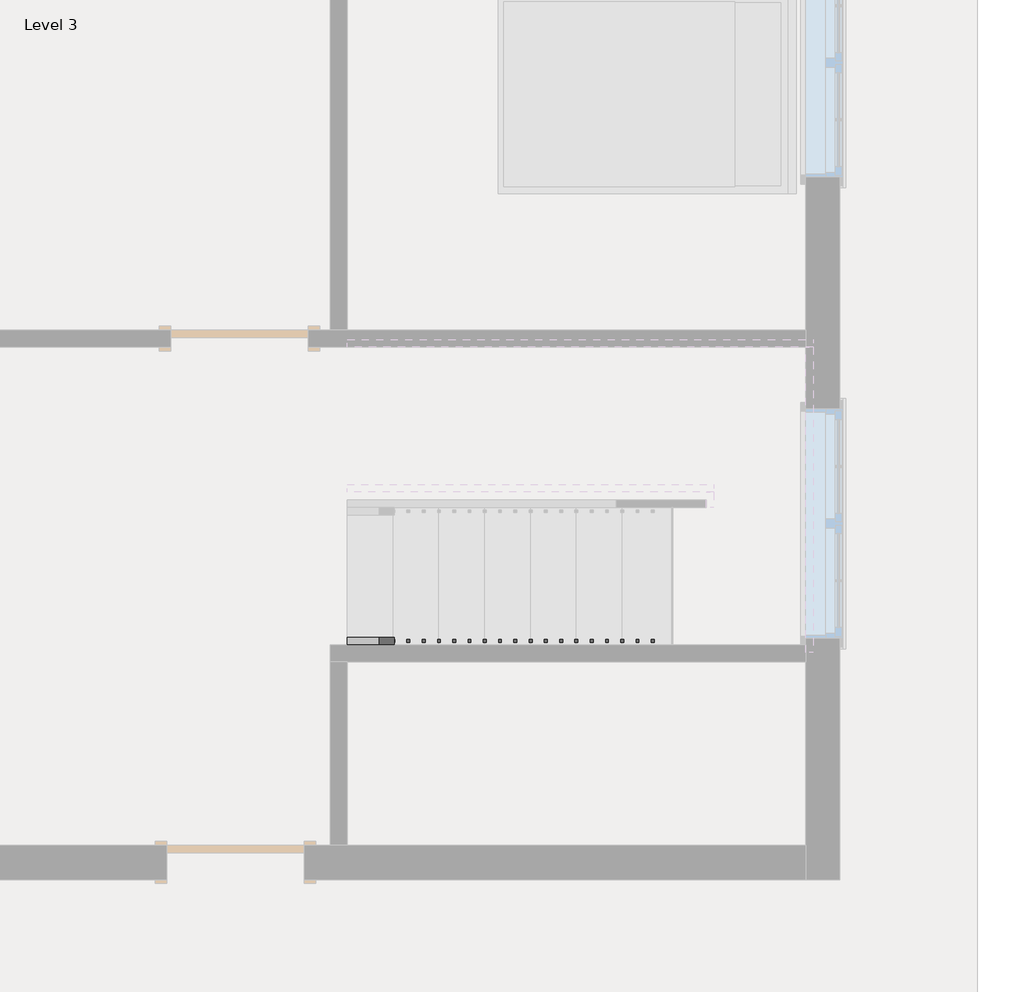
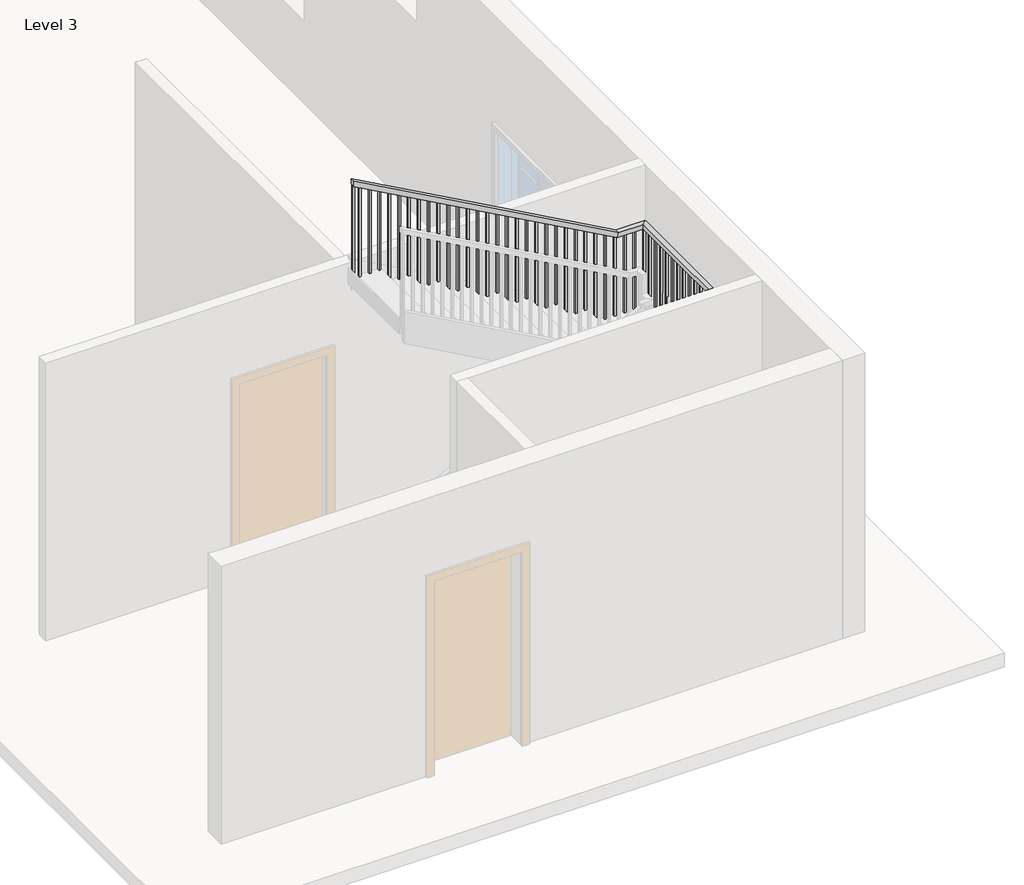
# One storey, part 2 of 3: 1 railing.
"""IFC4 building model written with IfcOpenShell, lengths in millimetres."""

from ifc_helpers import new_model, si_unit, frame, origin, place, context, project, spatial, polyline, outline, extrude, faceted_brep, element, save

model = new_model("IFC4")

# Units and contexts
model_context = context("Model", 3, world=origin())
ifc_project = project(units=[si_unit("LENGTHUNIT", "METRE", prefix="MILLI")], contexts=[model_context])

# Site, building, storey
site = spatial("IfcSite", under=ifc_project)
building = spatial("IfcBuilding", under=site)
storey = spatial("IfcBuildingStorey", under=building, Name="Level 3", Elevation=6248.4)

# Railing
placement = place(None, origin())
element("IfcRailing", 1, ObjectType="Handrail - Rectangular", at=placement, inside=storey, context=model_context, shape_type="SolidModel", body=[
    faceted_brep([(-1197.97188, -4765.70869, 7332.1333333), (-1197.97188, -4765.70869, 7274.020221), (-1197.97188, -4816.50869, 7274.020221), (-1197.97188, -4816.50869, 7332.1333333), (1240.42812, -4765.70869, 8686.8), (1253.5917222, -4765.70869, 8636.0), (1253.5917222, -4816.50869, 8636.0), (1240.42812, -4816.50869, 8686.8), (1799.22812, -4765.70869, 8686.8), (1799.22812, -4765.70869, 8636.0), (1850.02812, -4816.50869, 8636.0), (1850.02812, -4816.50869, 8686.8), (1799.22812, -2886.10869, 8686.8), (1799.22812, -2886.10869, 8636.0), (1850.02812, -2835.30869, 8636.0), (1850.02812, -2835.30869, 8686.8), (1545.22812, -2886.10869, 8686.8), (1532.0645177, -2886.10869, 8636.0), (1532.0645177, -2835.30869, 8636.0), (1545.22812, -2835.30869, 8686.8), (-1197.97188, -2886.10869, 10210.8), (-1197.97188, -2835.30869, 10210.8), (-1197.97188, -2835.30869, 10152.6868876), (-1197.97188, -2886.10869, 10152.6868876)], [[[0, 1, 2, 3]], [[1, 0, 4, 5]], [[2, 1, 5, 6]], [[3, 2, 6, 7]], [[0, 3, 7, 4]], [[5, 4, 8, 9]], [[6, 5, 9, 10]], [[7, 6, 10, 11]], [[4, 7, 11, 8]], [[9, 8, 12, 13]], [[10, 9, 13, 14]], [[11, 10, 14, 15]], [[8, 11, 15, 12]], [[13, 12, 16, 17]], [[14, 13, 17, 18]], [[15, 14, 18, 19]], [[12, 15, 19, 16]], [[20, 21, 22, 23]], [[17, 16, 20, 23]], [[18, 17, 23, 22]], [[19, 18, 22, 21]], [[16, 19, 21, 20]]]),
    extrude(outline(polyline([(10105.0618876, -1112.24688), (10115.645221, -1131.29688), (9127.0666667, -1131.29688), (9127.0666667, -1112.24688), (10105.0618876, -1112.24688)])), frame((0.0, -2870.23369, 0.0), z_axis=(0.0, 1.0, 0.0), x_axis=(0.0, 0.0, 1.0)), (0.0, 0.0, 1.0), 19.05),
    extrude(outline(polyline([(10048.6174432, -1010.64688), (10059.2007765, -1029.69688), (9127.0666667, -1029.69688), (9127.0666667, -1010.64688), (10048.6174432, -1010.64688)])), frame((0.0, -2870.23369, 0.0), z_axis=(0.0, 1.0, 0.0), x_axis=(0.0, 0.0, 1.0)), (0.0, 0.0, 1.0), 19.05),
    extrude(outline(polyline([(9992.1729988, -909.04688), (10002.7563321, -928.09688), (9127.0666667, -928.09688), (9127.0666667, -909.04688), (9992.1729988, -909.04688)])), frame((0.0, -2870.23369, 0.0), z_axis=(0.0, 1.0, 0.0), x_axis=(0.0, 0.0, 1.0)), (0.0, 0.0, 1.0), 19.05),
    extrude(outline(polyline([(9935.7285543, -807.44688), (9946.3118876, -826.49688), (8957.7333333, -826.49688), (8957.7333333, -807.44688), (9935.7285543, -807.44688)])), frame((0.0, -2870.23369, 0.0), z_axis=(0.0, 1.0, 0.0), x_axis=(0.0, 0.0, 1.0)), (0.0, 0.0, 1.0), 19.05),
    extrude(outline(polyline([(9879.2841099, -705.84688), (9889.8674432, -724.89688), (8957.7333333, -724.89688), (8957.7333333, -705.84688), (9879.2841099, -705.84688)])), frame((0.0, -2870.23369, 0.0), z_axis=(0.0, 1.0, 0.0), x_axis=(0.0, 0.0, 1.0)), (0.0, 0.0, 1.0), 19.05),
    extrude(outline(polyline([(9822.8396654, -604.24688), (9833.4229988, -623.29688), (8957.7333333, -623.29688), (8957.7333333, -604.24688), (9822.8396654, -604.24688)])), frame((0.0, -2870.23369, 0.0), z_axis=(0.0, 1.0, 0.0), x_axis=(0.0, 0.0, 1.0)), (0.0, 0.0, 1.0), 19.05),
    extrude(outline(polyline([(9766.395221, -502.64688), (9776.9785543, -521.69688), (8788.4, -521.69688), (8788.4, -502.64688), (9766.395221, -502.64688)])), frame((0.0, -2870.23369, 0.0), z_axis=(0.0, 1.0, 0.0), x_axis=(0.0, 0.0, 1.0)), (0.0, 0.0, 1.0), 19.05),
    extrude(outline(polyline([(9709.9507765, -401.04688), (9720.5341099, -420.09688), (8788.4, -420.09688), (8788.4, -401.04688), (9709.9507765, -401.04688)])), frame((0.0, -2870.23369, 0.0), z_axis=(0.0, 1.0, 0.0), x_axis=(0.0, 0.0, 1.0)), (0.0, 0.0, 1.0), 19.05),
    extrude(outline(polyline([(9653.5063321, -299.44688), (9664.0896654, -318.49688), (8788.4, -318.49688), (8788.4, -299.44688), (9653.5063321, -299.44688)])), frame((0.0, -2870.23369, 0.0), z_axis=(0.0, 1.0, 0.0), x_axis=(0.0, 0.0, 1.0)), (0.0, 0.0, 1.0), 19.05),
    extrude(outline(polyline([(9597.0618876, -197.84688), (9607.645221, -216.89688), (8619.0666667, -216.89688), (8619.0666667, -197.84688), (9597.0618876, -197.84688)])), frame((0.0, -2870.23369, 0.0), z_axis=(0.0, 1.0, 0.0), x_axis=(0.0, 0.0, 1.0)), (0.0, 0.0, 1.0), 19.05),
    extrude(outline(polyline([(9540.6174432, -96.24688), (9551.2007765, -115.29688), (8619.0666667, -115.29688), (8619.0666667, -96.24688), (9540.6174432, -96.24688)])), frame((0.0, -2870.23369, 0.0), z_axis=(0.0, 1.0, 0.0), x_axis=(0.0, 0.0, 1.0)), (0.0, 0.0, 1.0), 19.05),
    extrude(outline(polyline([(9484.1729988, 5.35312), (9494.7563321, -13.69688), (8619.0666667, -13.69688), (8619.0666667, 5.35312), (9484.1729988, 5.35312)])), frame((0.0, -2870.23369, 0.0), z_axis=(0.0, 1.0, 0.0), x_axis=(0.0, 0.0, 1.0)), (0.0, 0.0, 1.0), 19.05),
    extrude(outline(polyline([(9427.7285543, 106.95312), (9438.3118876, 87.90312), (8449.7333333, 87.90312), (8449.7333333, 106.95312), (9427.7285543, 106.95312)])), frame((0.0, -2870.23369, 0.0), z_axis=(0.0, 1.0, 0.0), x_axis=(0.0, 0.0, 1.0)), (0.0, 0.0, 1.0), 19.05),
    extrude(outline(polyline([(9371.2841099, 208.55312), (9381.8674432, 189.50312), (8449.7333333, 189.50312), (8449.7333333, 208.55312), (9371.2841099, 208.55312)])), frame((0.0, -2870.23369, 0.0), z_axis=(0.0, 1.0, 0.0), x_axis=(0.0, 0.0, 1.0)), (0.0, 0.0, 1.0), 19.05),
    extrude(outline(polyline([(9314.8396654, 310.15312), (9325.4229988, 291.10312), (8449.7333333, 291.10312), (8449.7333333, 310.15312), (9314.8396654, 310.15312)])), frame((0.0, -2870.23369, 0.0), z_axis=(0.0, 1.0, 0.0), x_axis=(0.0, 0.0, 1.0)), (0.0, 0.0, 1.0), 19.05),
    extrude(outline(polyline([(9258.395221, 411.75312), (9268.9785543, 392.70312), (8280.4, 392.70312), (8280.4, 411.75312), (9258.395221, 411.75312)])), frame((0.0, -2870.23369, 0.0), z_axis=(0.0, 1.0, 0.0), x_axis=(0.0, 0.0, 1.0)), (0.0, 0.0, 1.0), 19.05),
    extrude(outline(polyline([(9201.9507765, 513.35312), (9212.5341099, 494.30312), (8280.4, 494.30312), (8280.4, 513.35312), (9201.9507765, 513.35312)])), frame((0.0, -2870.23369, 0.0), z_axis=(0.0, 1.0, 0.0), x_axis=(0.0, 0.0, 1.0)), (0.0, 0.0, 1.0), 19.05),
    extrude(outline(polyline([(9145.5063321, 614.95312), (9156.0896654, 595.90312), (8280.4, 595.90312), (8280.4, 614.95312), (9145.5063321, 614.95312)])), frame((0.0, -2870.23369, 0.0), z_axis=(0.0, 1.0, 0.0), x_axis=(0.0, 0.0, 1.0)), (0.0, 0.0, 1.0), 19.05),
    extrude(outline(polyline([(9089.0618876, 716.55312), (9099.645221, 697.50312), (8111.0666667, 697.50312), (8111.0666667, 716.55312), (9089.0618876, 716.55312)])), frame((0.0, -2870.23369, 0.0), z_axis=(0.0, 1.0, 0.0), x_axis=(0.0, 0.0, 1.0)), (0.0, 0.0, 1.0), 19.05),
    extrude(outline(polyline([(9032.6174432, 818.15312), (9043.2007765, 799.10312), (8111.0666667, 799.10312), (8111.0666667, 818.15312), (9032.6174432, 818.15312)])), frame((0.0, -2870.23369, 0.0), z_axis=(0.0, 1.0, 0.0), x_axis=(0.0, 0.0, 1.0)), (0.0, 0.0, 1.0), 19.05),
    extrude(outline(polyline([(8976.1729988, 919.75312), (8986.7563321, 900.70312), (8111.0666667, 900.70312), (8111.0666667, 919.75312), (8976.1729988, 919.75312)])), frame((0.0, -2870.23369, 0.0), z_axis=(0.0, 1.0, 0.0), x_axis=(0.0, 0.0, 1.0)), (0.0, 0.0, 1.0), 19.05),
    extrude(outline(polyline([(8919.7285543, 1021.35312), (8930.3118876, 1002.30312), (7941.7333333, 1002.30312), (7941.7333333, 1021.35312), (8919.7285543, 1021.35312)])), frame((0.0, -2870.23369, 0.0), z_axis=(0.0, 1.0, 0.0), x_axis=(0.0, 0.0, 1.0)), (0.0, 0.0, 1.0), 19.05),
    extrude(outline(polyline([(8863.2841099, 1122.95312), (8873.8674432, 1103.90312), (7941.7333333, 1103.90312), (7941.7333333, 1122.95312), (8863.2841099, 1122.95312)])), frame((0.0, -2870.23369, 0.0), z_axis=(0.0, 1.0, 0.0), x_axis=(0.0, 0.0, 1.0)), (0.0, 0.0, 1.0), 19.05),
    extrude(outline(polyline([(8806.8396654, 1224.55312), (8817.4229988, 1205.50312), (7941.7333333, 1205.50312), (7941.7333333, 1224.55312), (8806.8396654, 1224.55312)])), frame((0.0, -2870.23369, 0.0), z_axis=(0.0, 1.0, 0.0), x_axis=(0.0, 0.0, 1.0)), (0.0, 0.0, 1.0), 19.05),
    extrude(outline(polyline([(8750.395221, 1326.15312), (8760.9785543, 1307.10312), (7772.4, 1307.10312), (7772.4, 1326.15312), (8750.395221, 1326.15312)])), frame((0.0, -2870.23369, 0.0), z_axis=(0.0, 1.0, 0.0), x_axis=(0.0, 0.0, 1.0)), (0.0, 0.0, 1.0), 19.05),
    extrude(outline(polyline([(8693.9507765, 1427.75312), (8704.5341099, 1408.70312), (7772.4, 1408.70312), (7772.4, 1427.75312), (8693.9507765, 1427.75312)])), frame((0.0, -2870.23369, 0.0), z_axis=(0.0, 1.0, 0.0), x_axis=(0.0, 0.0, 1.0)), (0.0, 0.0, 1.0), 19.05),
    extrude(outline(polyline([(8637.5063321, 1529.35312), (8648.0896654, 1510.30312), (7772.4, 1510.30312), (7772.4, 1529.35312), (8637.5063321, 1529.35312)])), frame((0.0, -2870.23369, 0.0), z_axis=(0.0, 1.0, 0.0), x_axis=(0.0, 0.0, 1.0)), (0.0, 0.0, 1.0), 19.05),
    extrude(outline(polyline([(1630.95312, -2851.18369), (1630.95312, -2870.23369), (1611.90312, -2870.23369), (1611.90312, -2851.18369), (1630.95312, -2851.18369)])), frame((0.0, 0.0, 7772.4), z_axis=(0.0, 0.0, 1.0), x_axis=(1.0, 0.0, 0.0)), (0.0, 0.0, 1.0), 863.6),
    extrude(outline(polyline([(1732.55312, -2851.18369), (1732.55312, -2870.23369), (1713.50312, -2870.23369), (1713.50312, -2851.18369), (1732.55312, -2851.18369)])), frame((0.0, 0.0, 7772.4), z_axis=(0.0, 0.0, 1.0), x_axis=(1.0, 0.0, 0.0)), (0.0, 0.0, 1.0), 863.6),
    extrude(outline(polyline([(1834.15312, -2971.83369), (1815.10312, -2971.83369), (1815.10312, -2952.78369), (1834.15312, -2952.78369), (1834.15312, -2971.83369)])), frame((0.0, 0.0, 7772.4), z_axis=(0.0, 0.0, 1.0), x_axis=(1.0, 0.0, 0.0)), (0.0, 0.0, 1.0), 863.6),
    extrude(outline(polyline([(1834.15312, -3073.43369), (1815.10312, -3073.43369), (1815.10312, -3054.38369), (1834.15312, -3054.38369), (1834.15312, -3073.43369)])), frame((0.0, 0.0, 7772.4), z_axis=(0.0, 0.0, 1.0), x_axis=(1.0, 0.0, 0.0)), (0.0, 0.0, 1.0), 863.6),
    extrude(outline(polyline([(1834.15312, -3175.03369), (1815.10312, -3175.03369), (1815.10312, -3155.98369), (1834.15312, -3155.98369), (1834.15312, -3175.03369)])), frame((0.0, 0.0, 7772.4), z_axis=(0.0, 0.0, 1.0), x_axis=(1.0, 0.0, 0.0)), (0.0, 0.0, 1.0), 863.6),
    extrude(outline(polyline([(1834.15312, -3276.63369), (1815.10312, -3276.63369), (1815.10312, -3257.58369), (1834.15312, -3257.58369), (1834.15312, -3276.63369)])), frame((0.0, 0.0, 7772.4), z_axis=(0.0, 0.0, 1.0), x_axis=(1.0, 0.0, 0.0)), (0.0, 0.0, 1.0), 863.6),
    extrude(outline(polyline([(1834.15312, -3378.23369), (1815.10312, -3378.23369), (1815.10312, -3359.18369), (1834.15312, -3359.18369), (1834.15312, -3378.23369)])), frame((0.0, 0.0, 7772.4), z_axis=(0.0, 0.0, 1.0), x_axis=(1.0, 0.0, 0.0)), (0.0, 0.0, 1.0), 863.6),
    extrude(outline(polyline([(1834.15312, -3479.83369), (1815.10312, -3479.83369), (1815.10312, -3460.78369), (1834.15312, -3460.78369), (1834.15312, -3479.83369)])), frame((0.0, 0.0, 7772.4), z_axis=(0.0, 0.0, 1.0), x_axis=(1.0, 0.0, 0.0)), (0.0, 0.0, 1.0), 863.6),
    extrude(outline(polyline([(1834.15312, -3581.43369), (1815.10312, -3581.43369), (1815.10312, -3562.38369), (1834.15312, -3562.38369), (1834.15312, -3581.43369)])), frame((0.0, 0.0, 7772.4), z_axis=(0.0, 0.0, 1.0), x_axis=(1.0, 0.0, 0.0)), (0.0, 0.0, 1.0), 863.6),
    extrude(outline(polyline([(1834.15312, -3683.03369), (1815.10312, -3683.03369), (1815.10312, -3663.98369), (1834.15312, -3663.98369), (1834.15312, -3683.03369)])), frame((0.0, 0.0, 7772.4), z_axis=(0.0, 0.0, 1.0), x_axis=(1.0, 0.0, 0.0)), (0.0, 0.0, 1.0), 863.6),
    extrude(outline(polyline([(1834.15312, -3784.63369), (1815.10312, -3784.63369), (1815.10312, -3765.58369), (1834.15312, -3765.58369), (1834.15312, -3784.63369)])), frame((0.0, 0.0, 7772.4), z_axis=(0.0, 0.0, 1.0), x_axis=(1.0, 0.0, 0.0)), (0.0, 0.0, 1.0), 863.6),
    extrude(outline(polyline([(1834.15312, -3886.23369), (1815.10312, -3886.23369), (1815.10312, -3867.18369), (1834.15312, -3867.18369), (1834.15312, -3886.23369)])), frame((0.0, 0.0, 7772.4), z_axis=(0.0, 0.0, 1.0), x_axis=(1.0, 0.0, 0.0)), (0.0, 0.0, 1.0), 863.6),
    extrude(outline(polyline([(1834.15312, -3987.83369), (1815.10312, -3987.83369), (1815.10312, -3968.78369), (1834.15312, -3968.78369), (1834.15312, -3987.83369)])), frame((0.0, 0.0, 7772.4), z_axis=(0.0, 0.0, 1.0), x_axis=(1.0, 0.0, 0.0)), (0.0, 0.0, 1.0), 863.6),
    extrude(outline(polyline([(1834.15312, -4089.43369), (1815.10312, -4089.43369), (1815.10312, -4070.38369), (1834.15312, -4070.38369), (1834.15312, -4089.43369)])), frame((0.0, 0.0, 7772.4), z_axis=(0.0, 0.0, 1.0), x_axis=(1.0, 0.0, 0.0)), (0.0, 0.0, 1.0), 863.6),
    extrude(outline(polyline([(1834.15312, -4191.03369), (1815.10312, -4191.03369), (1815.10312, -4171.98369), (1834.15312, -4171.98369), (1834.15312, -4191.03369)])), frame((0.0, 0.0, 7772.4), z_axis=(0.0, 0.0, 1.0), x_axis=(1.0, 0.0, 0.0)), (0.0, 0.0, 1.0), 863.6),
    extrude(outline(polyline([(1834.15312, -4292.63369), (1815.10312, -4292.63369), (1815.10312, -4273.58369), (1834.15312, -4273.58369), (1834.15312, -4292.63369)])), frame((0.0, 0.0, 7772.4), z_axis=(0.0, 0.0, 1.0), x_axis=(1.0, 0.0, 0.0)), (0.0, 0.0, 1.0), 863.6),
    extrude(outline(polyline([(1834.15312, -4394.23369), (1815.10312, -4394.23369), (1815.10312, -4375.18369), (1834.15312, -4375.18369), (1834.15312, -4394.23369)])), frame((0.0, 0.0, 7772.4), z_axis=(0.0, 0.0, 1.0), x_axis=(1.0, 0.0, 0.0)), (0.0, 0.0, 1.0), 863.6),
    extrude(outline(polyline([(1834.15312, -4495.83369), (1815.10312, -4495.83369), (1815.10312, -4476.78369), (1834.15312, -4476.78369), (1834.15312, -4495.83369)])), frame((0.0, 0.0, 7772.4), z_axis=(0.0, 0.0, 1.0), x_axis=(1.0, 0.0, 0.0)), (0.0, 0.0, 1.0), 863.6),
    extrude(outline(polyline([(1834.15312, -4597.43369), (1815.10312, -4597.43369), (1815.10312, -4578.38369), (1834.15312, -4578.38369), (1834.15312, -4597.43369)])), frame((0.0, 0.0, 7772.4), z_axis=(0.0, 0.0, 1.0), x_axis=(1.0, 0.0, 0.0)), (0.0, 0.0, 1.0), 863.6),
    extrude(outline(polyline([(1834.15312, -4699.03369), (1815.10312, -4699.03369), (1815.10312, -4679.98369), (1834.15312, -4679.98369), (1834.15312, -4699.03369)])), frame((0.0, 0.0, 7772.4), z_axis=(0.0, 0.0, 1.0), x_axis=(1.0, 0.0, 0.0)), (0.0, 0.0, 1.0), 863.6),
    extrude(outline(polyline([(1738.90312, -4800.63369), (1738.90312, -4781.58369), (1757.95312, -4781.58369), (1757.95312, -4800.63369), (1738.90312, -4800.63369)])), frame((0.0, 0.0, 7772.4), z_axis=(0.0, 0.0, 1.0), x_axis=(1.0, 0.0, 0.0)), (0.0, 0.0, 1.0), 863.6),
    extrude(outline(polyline([(1637.30312, -4800.63369), (1637.30312, -4781.58369), (1656.35312, -4781.58369), (1656.35312, -4800.63369), (1637.30312, -4800.63369)])), frame((0.0, 0.0, 7772.4), z_axis=(0.0, 0.0, 1.0), x_axis=(1.0, 0.0, 0.0)), (0.0, 0.0, 1.0), 863.6),
    extrude(outline(polyline([(1535.70312, -4800.63369), (1535.70312, -4781.58369), (1554.75312, -4781.58369), (1554.75312, -4800.63369), (1535.70312, -4800.63369)])), frame((0.0, 0.0, 7772.4), z_axis=(0.0, 0.0, 1.0), x_axis=(1.0, 0.0, 0.0)), (0.0, 0.0, 1.0), 863.6),
    extrude(outline(polyline([(1434.10312, -4800.63369), (1434.10312, -4781.58369), (1453.15312, -4781.58369), (1453.15312, -4800.63369), (1434.10312, -4800.63369)])), frame((0.0, 0.0, 7772.4), z_axis=(0.0, 0.0, 1.0), x_axis=(1.0, 0.0, 0.0)), (0.0, 0.0, 1.0), 863.6),
    extrude(outline(polyline([(1332.50312, -4800.63369), (1332.50312, -4781.58369), (1351.55312, -4781.58369), (1351.55312, -4800.63369), (1332.50312, -4800.63369)])), frame((0.0, 0.0, 7772.4), z_axis=(0.0, 0.0, 1.0), x_axis=(1.0, 0.0, 0.0)), (0.0, 0.0, 1.0), 863.6),
    extrude(outline(polyline([(8633.9785543, 1249.95312), (8623.395221, 1230.90312), (7772.4, 1230.90312), (7772.4, 1249.95312), (8633.9785543, 1249.95312)])), frame((0.0, -4800.63369, 0.0), z_axis=(0.0, 1.0, 0.0), x_axis=(0.0, 0.0, 1.0)), (0.0, 0.0, 1.0), 19.05),
    extrude(outline(polyline([(8577.5341099, 1148.35312), (8566.9507765, 1129.30312), (7603.0666667, 1129.30312), (7603.0666667, 1148.35312), (8577.5341099, 1148.35312)])), frame((0.0, -4800.63369, 0.0), z_axis=(0.0, 1.0, 0.0), x_axis=(0.0, 0.0, 1.0)), (0.0, 0.0, 1.0), 19.05),
    extrude(outline(polyline([(8521.0896654, 1046.75312), (8510.5063321, 1027.70312), (7603.0666667, 1027.70312), (7603.0666667, 1046.75312), (8521.0896654, 1046.75312)])), frame((0.0, -4800.63369, 0.0), z_axis=(0.0, 1.0, 0.0), x_axis=(0.0, 0.0, 1.0)), (0.0, 0.0, 1.0), 19.05),
    extrude(outline(polyline([(8464.645221, 945.15312), (8454.0618876, 926.10312), (7603.0666667, 926.10312), (7603.0666667, 945.15312), (8464.645221, 945.15312)])), frame((0.0, -4800.63369, 0.0), z_axis=(0.0, 1.0, 0.0), x_axis=(0.0, 0.0, 1.0)), (0.0, 0.0, 1.0), 19.05),
    extrude(outline(polyline([(8408.2007765, 843.55312), (8397.6174432, 824.50312), (7433.7333333, 824.50312), (7433.7333333, 843.55312), (8408.2007765, 843.55312)])), frame((0.0, -4800.63369, 0.0), z_axis=(0.0, 1.0, 0.0), x_axis=(0.0, 0.0, 1.0)), (0.0, 0.0, 1.0), 19.05),
    extrude(outline(polyline([(8351.7563321, 741.95312), (8341.1729988, 722.90312), (7433.7333333, 722.90312), (7433.7333333, 741.95312), (8351.7563321, 741.95312)])), frame((0.0, -4800.63369, 0.0), z_axis=(0.0, 1.0, 0.0), x_axis=(0.0, 0.0, 1.0)), (0.0, 0.0, 1.0), 19.05),
    extrude(outline(polyline([(8295.3118876, 640.35312), (8284.7285543, 621.30312), (7433.7333333, 621.30312), (7433.7333333, 640.35312), (8295.3118876, 640.35312)])), frame((0.0, -4800.63369, 0.0), z_axis=(0.0, 1.0, 0.0), x_axis=(0.0, 0.0, 1.0)), (0.0, 0.0, 1.0), 19.05),
    extrude(outline(polyline([(8238.8674432, 538.75312), (8228.2841099, 519.70312), (7264.4, 519.70312), (7264.4, 538.75312), (8238.8674432, 538.75312)])), frame((0.0, -4800.63369, 0.0), z_axis=(0.0, 1.0, 0.0), x_axis=(0.0, 0.0, 1.0)), (0.0, 0.0, 1.0), 19.05),
    extrude(outline(polyline([(8182.4229988, 437.15312), (8171.8396654, 418.10312), (7264.4, 418.10312), (7264.4, 437.15312), (8182.4229988, 437.15312)])), frame((0.0, -4800.63369, 0.0), z_axis=(0.0, 1.0, 0.0), x_axis=(0.0, 0.0, 1.0)), (0.0, 0.0, 1.0), 19.05),
    extrude(outline(polyline([(8125.9785543, 335.55312), (8115.395221, 316.50312), (7264.4, 316.50312), (7264.4, 335.55312), (8125.9785543, 335.55312)])), frame((0.0, -4800.63369, 0.0), z_axis=(0.0, 1.0, 0.0), x_axis=(0.0, 0.0, 1.0)), (0.0, 0.0, 1.0), 19.05),
    extrude(outline(polyline([(8069.5341099, 233.95312), (8058.9507765, 214.90312), (7095.0666667, 214.90312), (7095.0666667, 233.95312), (8069.5341099, 233.95312)])), frame((0.0, -4800.63369, 0.0), z_axis=(0.0, 1.0, 0.0), x_axis=(0.0, 0.0, 1.0)), (0.0, 0.0, 1.0), 19.05),
    extrude(outline(polyline([(8013.0896654, 132.35312), (8002.5063321, 113.30312), (7095.0666667, 113.30312), (7095.0666667, 132.35312), (8013.0896654, 132.35312)])), frame((0.0, -4800.63369, 0.0), z_axis=(0.0, 1.0, 0.0), x_axis=(0.0, 0.0, 1.0)), (0.0, 0.0, 1.0), 19.05),
    extrude(outline(polyline([(7956.645221, 30.75312), (7946.0618876, 11.70312), (7095.0666667, 11.70312), (7095.0666667, 30.75312), (7956.645221, 30.75312)])), frame((0.0, -4800.63369, 0.0), z_axis=(0.0, 1.0, 0.0), x_axis=(0.0, 0.0, 1.0)), (0.0, 0.0, 1.0), 19.05),
    extrude(outline(polyline([(7900.2007765, -70.84688), (7889.6174432, -89.89688), (6925.7333333, -89.89688), (6925.7333333, -70.84688), (7900.2007765, -70.84688)])), frame((0.0, -4800.63369, 0.0), z_axis=(0.0, 1.0, 0.0), x_axis=(0.0, 0.0, 1.0)), (0.0, 0.0, 1.0), 19.05),
    extrude(outline(polyline([(7843.7563321, -172.44688), (7833.1729988, -191.49688), (6925.7333333, -191.49688), (6925.7333333, -172.44688), (7843.7563321, -172.44688)])), frame((0.0, -4800.63369, 0.0), z_axis=(0.0, 1.0, 0.0), x_axis=(0.0, 0.0, 1.0)), (0.0, 0.0, 1.0), 19.05),
    extrude(outline(polyline([(7787.3118876, -274.04688), (7776.7285543, -293.09688), (6925.7333333, -293.09688), (6925.7333333, -274.04688), (7787.3118876, -274.04688)])), frame((0.0, -4800.63369, 0.0), z_axis=(0.0, 1.0, 0.0), x_axis=(0.0, 0.0, 1.0)), (0.0, 0.0, 1.0), 19.05),
    extrude(outline(polyline([(7730.8674432, -375.64688), (7720.2841099, -394.69688), (6756.4, -394.69688), (6756.4, -375.64688), (7730.8674432, -375.64688)])), frame((0.0, -4800.63369, 0.0), z_axis=(0.0, 1.0, 0.0), x_axis=(0.0, 0.0, 1.0)), (0.0, 0.0, 1.0), 19.05),
    extrude(outline(polyline([(7674.4229988, -477.24688), (7663.8396654, -496.29688), (6756.4, -496.29688), (6756.4, -477.24688), (7674.4229988, -477.24688)])), frame((0.0, -4800.63369, 0.0), z_axis=(0.0, 1.0, 0.0), x_axis=(0.0, 0.0, 1.0)), (0.0, 0.0, 1.0), 19.05),
    extrude(outline(polyline([(7617.9785543, -578.84688), (7607.395221, -597.89688), (6756.4, -597.89688), (6756.4, -578.84688), (7617.9785543, -578.84688)])), frame((0.0, -4800.63369, 0.0), z_axis=(0.0, 1.0, 0.0), x_axis=(0.0, 0.0, 1.0)), (0.0, 0.0, 1.0), 19.05),
    extrude(outline(polyline([(7561.5341099, -680.44688), (7550.9507765, -699.49688), (6587.0666667, -699.49688), (6587.0666667, -680.44688), (7561.5341099, -680.44688)])), frame((0.0, -4800.63369, 0.0), z_axis=(0.0, 1.0, 0.0), x_axis=(0.0, 0.0, 1.0)), (0.0, 0.0, 1.0), 19.05),
    extrude(outline(polyline([(7505.0896654, -782.04688), (7494.5063321, -801.09688), (6587.0666667, -801.09688), (6587.0666667, -782.04688), (7505.0896654, -782.04688)])), frame((0.0, -4800.63369, 0.0), z_axis=(0.0, 1.0, 0.0), x_axis=(0.0, 0.0, 1.0)), (0.0, 0.0, 1.0), 19.05),
    extrude(outline(polyline([(7448.645221, -883.64688), (7438.0618876, -902.69688), (6587.0666667, -902.69688), (6587.0666667, -883.64688), (7448.645221, -883.64688)])), frame((0.0, -4800.63369, 0.0), z_axis=(0.0, 1.0, 0.0), x_axis=(0.0, 0.0, 1.0)), (0.0, 0.0, 1.0), 19.05),
    extrude(outline(polyline([(7392.2007765, -985.24688), (7381.6174432, -1004.29688), (6417.7333333, -1004.29688), (6417.7333333, -985.24688), (7392.2007765, -985.24688)])), frame((0.0, -4800.63369, 0.0), z_axis=(0.0, 1.0, 0.0), x_axis=(0.0, 0.0, 1.0)), (0.0, 0.0, 1.0), 19.05),
    extrude(outline(polyline([(7335.7563321, -1086.84688), (7325.1729988, -1105.89688), (6417.7333333, -1105.89688), (6417.7333333, -1086.84688), (7335.7563321, -1086.84688)])), frame((0.0, -4800.63369, 0.0), z_axis=(0.0, 1.0, 0.0), x_axis=(0.0, 0.0, 1.0)), (0.0, 0.0, 1.0), 19.05),
    extrude(outline(polyline([(1834.15312, -2870.23369), (1815.10312, -2870.23369), (1815.10312, -2851.18369), (1834.15312, -2851.18369), (1834.15312, -2870.23369)])), frame((0.0, 0.0, 7772.4), z_axis=(0.0, 0.0, 1.0), x_axis=(1.0, 0.0, 0.0)), (0.0, 0.0, 1.0), 863.6),
    extrude(outline(polyline([(1815.10312, -4800.63369), (1815.10312, -4781.58369), (1834.15312, -4781.58369), (1834.15312, -4800.63369), (1815.10312, -4800.63369)])), frame((0.0, 0.0, 7772.4), z_axis=(0.0, 0.0, 1.0), x_axis=(1.0, 0.0, 0.0)), (0.0, 0.0, 1.0), 863.6),
    extrude(outline(polyline([(10142.1035543, -1178.92188), (10152.6868876, -1197.97188), (9127.0666667, -1197.97188), (9127.0666667, -1178.92188), (10142.1035543, -1178.92188)])), frame((0.0, -2870.23369, 0.0), z_axis=(0.0, 1.0, 0.0), x_axis=(0.0, 0.0, 1.0)), (0.0, 0.0, 1.0), 19.05),
    extrude(outline(polyline([(7284.6035543, -1178.92188), (7274.020221, -1197.97188), (6417.7333333, -1197.97188), (6417.7333333, -1178.92188), (7284.6035543, -1178.92188)])), frame((0.0, -4800.63369, 0.0), z_axis=(0.0, 1.0, 0.0), x_axis=(0.0, 0.0, 1.0)), (0.0, 0.0, 1.0), 19.05),
])

save(model, "model.ifc")

# Revit data of these elements
# Type "Handrail - Rectangular"
#   Assembly Code = "C2010400"
#   built-in parameter 1008612 = 0.0416667 (stored number, unit not read)
#   built-in parameter 1008611 = 0.0416667 (stored number, unit not read)
#   built-in parameter 1008609 = 0.333333 (stored number, unit not read)
#   built-in parameter 1008604 = 0.166667 (stored number, unit not read)
#   built-in parameter 1008603 = 0.166667 (stored number, unit not read)
#   Railing Height = 3' - 0"
#   built-in parameter 1008630 = 2
#   built-in parameter 1008610 = 2
#   built-in parameter 1008618 = Baluster - Square : 3/4"
# Element 1 (IfcRailing, "Handrail - Rectangular")
#   Phase Created = New Construction
